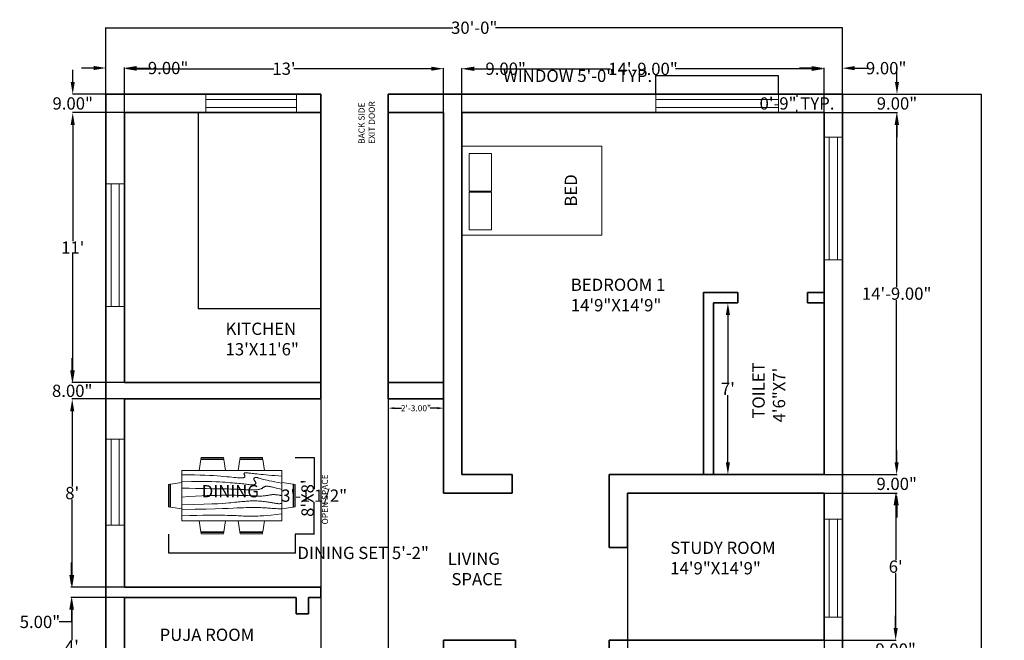
# Model space of a CAD drawing. Units: inches. Extents: x 14 to 1508, y -30 to 806.
# Tile 2 of 4: x 14 to 495, y 502 to 806. Entities that reach past the tile are written whole.
import ezdxf

# ---------------------------------------------------------------- set-up
doc = ezdxf.new("R2010")
doc.units = ezdxf.units.IN
doc.header["$MEASUREMENT"] = 0
for name, color, linetype, lineweight in [('A-ANNO-DIMS', 6, 'Continuous', 18), ('A-ANNO-TEXT', 7, 'Continuous', 18), ('A-AREA-IDEN', 3, 'Continuous', 18), ('A-FLOR-CASE', 8, 'Continuous', 25), ('A-FURN', 8, 'Continuous', 18), ('A-GLAZ', 4, 'Continuous', 18), ('A-WALL', 7, 'Continuous', 35)]:
    doc.layers.add(name, color=color, linetype=linetype, lineweight=lineweight)
doc.styles.get("Standard").update_dxf_attribs({"font": 'arial.ttf'})
doc.dimstyles.get("Standard").update_dxf_attribs({"dimtxt": 6, "dimasz": 0.18, "dimexe": 0.18, "dimexo": 0.0625, "dimgap": 0.09, "dimtad": 0, "dimtih": 1, "dimtoh": 1, "dimzin": 0, "dimdsep": 46, "dimlunit": 3, "dimtxsty": 'Standard', "dimcen": 0.09, "dimadec": 0, "dimazin": 0, "dimtfac": 1, "dimtofl": 0, "dimtmove": 0, "dimatfit": 3, "dimfxl": 1, "dimtolj": 1, "dimtzin": 0, "dimarcsym": 0})

# ---------------------------------------------------------------- blocks, each defined once
blk = doc.blocks.new('Dining Set - 36 x 72 in.')
for p, q in [((-22.2343, 26.00059), (-23.4847, 17.99762)), ((-22.2304, 26), (-5.7608, 26)), ((-22, 27.5), (-22.1562, 26.50042)), ((-5.8416, 26.5), (-22.1534, 26.5)), ((-22, 27.5), (-6, 27.5)), ((-5.8437, 26.49966), (-6, 27.5)), ((-4.5152, 17.99762), (-5.7655, 25.99926)), ((5.7657, 26.00059), (4.5153, 17.99762)), ((5.7696, 26), (22.2392, 26)), ((6, 27.5), (5.8438, 26.50042)), ((22.1584, 26.5), (5.8466, 26.5)), ((6, 27.5), (22, 27.5)), ((22.1563, 26.49966), (22, 27.5)), ((23.4848, 17.99762), (22.2345, 25.99926)), ((36, 18), (-36, 18)), ((-36, 18), (-36, -18)), ((36, -18), (36, 18)), ((-45.5, 8), (-44.5004, 8.15617)), ((-45.5, 8), (-45.5, -8)), ((-44.5, -8.15843), (-44.5, 8.15338)), ((-44.0006, 8.23428), (-35.9976, 9.48474)), ((-44, 8.23041), (-44, -8.23915)), ((44.0006, 8.23428), (35.9976, 9.48474)), ((44, 8.23041), (44, -8.23915)), ((44.5, -8.15843), (44.5, 8.15338)), ((45.5, 8), (44.5005, 8.15617)), ((45.5, 8), (45.5, -8)), ((-44.4997, -8.15631), (-45.5, -8)), ((-35.9976, -9.48476), (-43.9993, -8.2345)), ((35.9976, -9.48476), (43.9993, -8.2345)), ((44.4997, -8.15631), (45.5, -8)), ((-36, -18), (36, -18)), ((-22.2343, -26.0006), (-23.4847, -17.99762)), ((-4.5152, -17.99762), (-5.7655, -25.99928)), ((5.7657, -26.0006), (4.5153, -17.99762)), ((23.4848, -17.99762), (22.2345, -25.99928)), ((-22.2304, -26), (-5.7608, -26)), ((-22, -27.5), (-22.1562, -26.50044)), ((-5.8416, -26.5), (-22.1534, -26.5)), ((-22, -27.5), (-6, -27.5)), ((-5.8437, -26.49967), (-6, -27.5)), ((5.7696, -26), (22.2392, -26)), ((6, -27.5), (5.8438, -26.50044)), ((22.1584, -26.5), (5.8466, -26.5)), ((6, -27.5), (22, -27.5)), ((22.1563, -26.49967), (22, -27.5))]:
    blk.add_line(p, q)
for points in [[(-36, 15), (-31.1772, 14.97754), (-26.8079, 14.91406), (-22.8538, 14.81543), (-19.276, 14.6875), (-16.0362, 14.53613), (-13.0957, 14.36718), (-10.4159, 14.18652), (-7.9583, 14), (-5.6904, 13.81315), (-3.6035, 13.63021), (-1.6954, 13.45508), (0.0365, 13.29166), (1.5945, 13.14388), (2.9811, 13.01562), (4.1988, 12.9108), (5.25, 12.83333), (6.1393, 12.78613), (6.8802, 12.76823), (7.4883, 12.77767), (7.9792, 12.8125), (8.3685, 12.87077), (8.6719, 12.95052), (8.9049, 13.0498), (9.0833, 13.16666), (9.2205, 13.29899), (9.3216, 13.44401), (9.3895, 13.59879), (9.4271, 13.76041), (9.4373, 13.92594), (9.4232, 14.09245), (9.3875, 14.257), (9.3333, 14.41666), (9.2638, 14.56917), (9.1836, 14.71484), (9.0975, 14.85465), (9.0104, 14.98958), (8.9272, 15.1206), (8.8529, 15.2487), (8.7922, 15.37483), (8.75, 15.5), (8.7305, 15.62467), (8.7344, 15.74739), (8.7617, 15.86621), (8.8125, 15.97916), (8.8867, 16.08431), (8.9844, 16.17968), (9.1055, 16.26334), (9.25, 16.33333), (9.4189, 16.38802), (9.6172, 16.42708), (9.8506, 16.45052), (10.125, 16.45833), (10.4463, 16.45052), (10.8203, 16.42708), (11.2529, 16.38802), (11.75, 16.33333), (12.3184, 16.26318), (12.9694, 16.17838), (13.7151, 16.07991), (14.5677, 15.96875), (15.5395, 15.84586), (16.6426, 15.71224), (17.8893, 15.56884), (19.2917, 15.41666), (20.859, 15.25667), (22.5879, 15.08984), (24.4721, 14.91715), (26.5052, 14.73958), (28.6809, 14.5581), (30.9929, 14.3737), (33.4347, 14.18733), (36, 14)], [(-36, 10), (-28.9766, 10.14274), (-23.1725, 10.20442), (-18.4241, 10.19775), (-14.5677, 10.13541), (-11.4399, 10.03011), (-8.877, 9.89453), (-6.7154, 9.74137), (-4.7917, 9.58333), (-2.9698, 9.43082), (-1.2246, 9.28515), (0.4415, 9.14534), (2.026, 9.01041), (3.5266, 8.87939), (4.9408, 8.7513), (6.266, 8.62516), (7.5, 8.5), (8.6411, 8.37549), (9.6914, 8.2539), (10.6538, 8.13818), (11.5312, 8.03125), (12.3267, 7.93603), (13.043, 7.85547), (13.6831, 7.79248), (14.25, 7.75), (14.7471, 7.7303), (15.1797, 7.73307), (15.5537, 7.75732), (15.875, 7.80208), (16.1494, 7.86637), (16.3828, 7.94922), (16.5811, 8.04964), (16.75, 8.16666), (16.8944, 8.29915), (17.0143, 8.44531), (17.1089, 8.60319), (17.1771, 8.77083), (17.218, 8.94629), (17.2305, 9.1276), (17.2137, 9.31282), (17.1667, 9.5), (17.0895, 9.6875), (16.987, 9.875), (16.8649, 10.0625), (16.7292, 10.25), (16.5856, 10.4375), (16.4401, 10.625), (16.2985, 10.8125), (16.1667, 11), (16.05, 11.18733), (15.9518, 11.3737), (15.8752, 11.5581), (15.8229, 11.73958), (15.798, 11.91715), (15.8034, 12.08984), (15.842, 12.25667), (15.9167, 12.41666), (16.0295, 12.56836), (16.1784, 12.70833), (16.3605, 12.83268), (16.5729, 12.9375), (16.8127, 13.01888), (17.0768, 13.07291), (17.3625, 13.0957), (17.6667, 13.08333), (17.9894, 13.03312), (18.3418, 12.94726), (18.7382, 12.82918), (19.1927, 12.68229), (19.7195, 12.51001), (20.3327, 12.31575), (21.0465, 12.10294), (21.875, 11.875), (22.8357, 11.63354), (23.959, 11.37304), (25.2786, 11.08618), (26.8282, 10.76562), (28.6414, 10.40405), (30.752, 9.99414), (33.1936, 9.52856), (36, 9)], [(-36, 5.5), (-30.7157, 5.3348), (-26.069, 5.20963), (-21.9946, 5.11767), (-18.4271, 5.05208), (-15.3009, 5.00602), (-12.5508, 4.97265), (-10.1112, 4.94515), (-7.9167, 4.91666), (-5.909, 4.88167), (-4.0586, 4.83984), (-2.3429, 4.79215), (-0.7396, 4.73958), (0.7739, 4.6831), (2.22, 4.6237), (3.6213, 4.56233), (5, 4.5), (6.373, 4.43782), (7.7344, 4.3776), (9.0723, 4.32129), (10.375, 4.27083), (11.6309, 4.22819), (12.8281, 4.19531), (13.9551, 4.17415), (15, 4.16666), (15.954, 4.17448), (16.819, 4.19791), (17.6001, 4.23698), (18.3021, 4.29166), (18.9299, 4.36198), (19.4883, 4.44791), (19.9823, 4.54948), (20.4167, 4.66666), (20.7969, 4.79899), (21.1302, 4.94401), (21.4245, 5.09879), (21.6875, 5.26041), (21.9271, 5.42594), (22.1511, 5.59245), (22.3672, 5.757), (22.5834, 5.91666), (22.8065, 6.06868), (23.0404, 6.21093), (23.2879, 6.34147), (23.5521, 6.45833), (23.8358, 6.55957), (24.142, 6.64323), (24.4735, 6.70735), (24.8334, 6.75), (25.2235, 6.76969), (25.642, 6.76692), (26.0858, 6.74267), (26.5521, 6.69791), (27.0379, 6.63362), (27.5404, 6.55078), (28.0565, 6.45036), (28.5834, 6.33333), (29.1242, 6.19987), (29.7071, 6.04687), (30.3661, 5.87044), (31.1354, 5.66666), (32.0493, 5.43164), (33.142, 5.16146), (34.4475, 4.85221), (36, 4.5)], [(-36, -1), (-30.7915, -0.6591), (-26.0195, -0.38216), (-21.6519, -0.16284), (-17.6563, 0.00521), (-14.0005, 0.12833), (-10.6523, 0.21289), (-7.5796, 0.26522), (-4.75, 0.29166), (-2.134, 0.29793), (0.2878, 0.28711), (2.5317, 0.26163), (4.6146, 0.22396), (6.5529, 0.17651), (8.3633, 0.12174), (10.0623, 0.06209), (11.6667, 0), (13.1899, -0.06201), (14.6341, -0.1211), (15.9982, -0.17432), (17.2813, -0.21875), (18.4823, -0.25147), (19.6003, -0.26953), (20.6343, -0.27002), (21.5834, -0.25), (22.4481, -0.20768), (23.2357, -0.14584), (23.9549, -0.06836), (24.6146, 0.02083), (25.2235, 0.11784), (25.7904, 0.21875), (26.3241, 0.31966), (26.8334, 0.41666), (27.3265, 0.50618), (27.8099, 0.58593), (28.2894, 0.65397), (28.7709, 0.70833), (29.2601, 0.74707), (29.763, 0.76823), (30.2855, 0.76985), (30.8334, 0.75), (31.4088, 0.70784), (31.9994, 0.64713), (32.589, 0.57275), (33.1615, 0.48958), (33.7008, 0.4025), (34.1908, 0.3164), (34.6153, 0.23616), (34.9584, 0.16666), (35.2099, 0.11165), (35.3848, 0.07031), (35.504, 0.04069), (35.5886, 0.02083), (35.6594, 0.00879), (35.7377, 0.0026), (35.8442, 0.00032), (36, 0)], [(-36, -6.5), (-27.1843, -6.31267), (-20.084, -6.1263), (-14.469, -5.9419), (-10.1094, -5.76042), (-6.7752, -5.58285), (-4.2363, -5.41016), (-2.2629, -5.24333), (-0.625, -5.08334), (0.8708, -4.93099), (2.2715, -4.78646), (3.5872, -4.64974), (4.8281, -4.52084), (6.0046, -4.39974), (7.127, -4.28646), (8.2053, -4.18099), (9.25, -4.08334), (10.2705, -3.99382), (11.2734, -3.91407), (12.2647, -3.84603), (13.25, -3.79167), (14.2354, -3.75293), (15.2266, -3.73177), (16.2295, -3.73015), (17.25, -3.75), (18.2912, -3.79248), (19.3451, -3.85547), (20.4009, -3.93604), (21.4479, -4.03125), (22.4754, -4.13819), (23.4727, -4.25391), (24.4289, -4.37549), (25.3334, -4.5), (26.1785, -4.62492), (26.9694, -4.74935), (27.7145, -4.87281), (28.4219, -4.99479), (29.1, -5.11483), (29.7572, -5.23242), (30.4016, -5.34709), (31.0417, -5.45834), (31.6837, -5.56437), (32.3262, -5.65821), (32.9658, -5.73153), (33.599, -5.77604), (34.2224, -5.78345), (34.8327, -5.74545), (35.4264, -5.65373), (36, -5.5)], [(-36, -10), (-26.4022, -9.81299), (-18.4675, -9.62891), (-11.9839, -9.45069), (-6.7396, -9.28125), (-2.5226, -9.12354), (0.8789, -8.98047), (3.6769, -8.85498), (6.0833, -8.75), (8.2767, -8.66765), (10.3021, -8.60677), (12.1712, -8.56543), (13.8958, -8.54167), (15.4876, -8.53353), (16.9583, -8.53907), (18.3197, -8.55632), (19.5834, -8.58334), (20.7616, -8.61841), (21.8685, -8.66081), (22.9188, -8.71004), (23.9271, -8.76563), (24.9081, -8.82707), (25.8763, -8.89388), (26.8465, -8.96558), (27.8334, -9.04167), (28.8474, -9.12118), (29.8828, -9.20117), (30.93, -9.27824), (31.9792, -9.34896), (33.0205, -9.40991), (34.0443, -9.45768), (35.0407, -9.48885), (36, -9.5)], [(-36, -14.5), (-30.0881, -14.33513), (-25.0332, -14.21224), (-20.7312, -14.12647), (-17.0781, -14.07292), (-13.97, -14.04671), (-11.3027, -14.04297), (-8.9724, -14.05681), (-6.875, -14.08334), (-4.9224, -14.11833), (-3.0905, -14.16016), (-1.3709, -14.20785), (0.2448, -14.26042), (1.7647, -14.3169), (3.1973, -14.3763), (4.5507, -14.43767), (5.8333, -14.5), (7.0554, -14.5621), (8.235, -14.62175), (9.3922, -14.67652), (10.5469, -14.72396), (11.7192, -14.76164), (12.929, -14.78711), (14.1965, -14.79794), (15.5417, -14.79167), (16.9933, -14.76424), (18.6152, -14.70508), (20.4804, -14.60197), (22.6615, -14.44271), (25.2312, -14.21509), (28.2624, -13.9069), (31.8277, -13.50594), (36, -13)]]:
    blk.add_lwpolyline(points)
blk = doc.blocks.new('*D3')
at = {"layer": 'A-ANNO-DIMS', "color": 0, "lineweight": -2, "transparency": 16777216}
for p, q in [((193.96, 620), (193.96, 615.39)), ((220.96, 620), (220.96, 615.39)), ((196.96, 615.57), (200.45, 615.57)), ((217.96, 615.57), (214.48, 615.57))]:
    blk.add_line(p, q, dxfattribs=at)
at = {"layer": 'A-ANNO-DIMS', "color": 0, "transparency": 16777216}
for points in [[(196.96, 616.07), (196.96, 615.07), (193.96, 615.57)], [(217.96, 616.07), (217.96, 615.07), (220.96, 615.57)]]:
    blk.add_solid(points, dxfattribs=at)
at = {"layer": 'Defpoints', "color": 0, "transparency": 16777216}
for p in [(193.96, 620.06), (220.96, 620.06), (220.96, 615.57)]:
    blk.add_point(p, dxfattribs=at)
at = {"layer": 'A-ANNO-DIMS', "color": 0, "transparency": 16777216, "insert": (207.46, 615.57), "char_height": 3, "attachment_point": 5}
blk.add_mtext('\\A1;2\'-3.00"', dxfattribs=at)
blk = doc.blocks.new('*D4')
at = {"layer": 'A-ANNO-DIMS', "color": 0, "lineweight": -2, "transparency": 16777216}
for p, q in [((39.7, 775.06), (39.7, 781.06)), ((66.46, 769.06), (39.52, 769.06)), ((64.9, 760.06), (39.52, 760.06)), ((39.7, 754.06), (39.7, 748.06))]:
    blk.add_line(p, q, dxfattribs=at)
at = {"layer": 'A-ANNO-DIMS', "color": 0, "transparency": 16777216}
for points in [[(38.7, 775.06), (40.7, 775.06), (39.7, 769.06)], [(38.7, 754.06), (40.7, 754.06), (39.7, 760.06)]]:
    blk.add_solid(points, dxfattribs=at)
at = {"layer": 'Defpoints', "color": 0, "transparency": 16777216}
for p in [(66.52, 769.06), (39.7, 760.06), (64.96, 760.06)]:
    blk.add_point(p, dxfattribs=at)
at = {"layer": 'A-ANNO-DIMS', "color": 0, "transparency": 16777216, "insert": (39.7, 764.56), "char_height": 6, "attachment_point": 5}
blk.add_mtext('\\A1;9.00"', dxfattribs=at)
blk = doc.blocks.new('*D5')
at = {"layer": 'A-ANNO-DIMS', "color": 0, "lineweight": -2, "transparency": 16777216}
for p, q in [((64.9, 760.06), (39.52, 760.06)), ((39.7, 754.06), (39.7, 697.16)), ((39.7, 634.06), (39.7, 690.96)), ((64.9, 628.06), (39.52, 628.06))]:
    blk.add_line(p, q, dxfattribs=at)
at = {"layer": 'A-ANNO-DIMS', "color": 0, "transparency": 16777216}
for points in [[(38.7, 754.06), (40.7, 754.06), (39.7, 760.06)], [(38.7, 634.06), (40.7, 634.06), (39.7, 628.06)]]:
    blk.add_solid(points, dxfattribs=at)
at = {"layer": 'Defpoints', "color": 0, "transparency": 16777216}
for p in [(39.7, 760.06), (64.96, 760.06), (64.96, 628.06)]:
    blk.add_point(p, dxfattribs=at)
at = {"layer": 'A-ANNO-DIMS', "color": 0, "transparency": 16777216, "insert": (39.7, 694.06), "char_height": 6, "attachment_point": 5}
blk.add_mtext("\\A1;11'", dxfattribs=at)
blk = doc.blocks.new('*D6')
at = {"layer": 'A-ANNO-DIMS', "color": 0, "lineweight": -2, "transparency": 16777216}
for p, q in [((39.45, 634.06), (39.45, 640.06)), ((64.9, 628.06), (39.27, 628.06)), ((64.9, 620.06), (39.27, 620.06)), ((39.45, 614.06), (39.45, 608.06))]:
    blk.add_line(p, q, dxfattribs=at)
at = {"layer": 'A-ANNO-DIMS', "color": 0, "transparency": 16777216}
for points in [[(38.45, 634.06), (40.45, 634.06), (39.45, 628.06)], [(38.45, 614.06), (40.45, 614.06), (39.45, 620.06)]]:
    blk.add_solid(points, dxfattribs=at)
at = {"layer": 'Defpoints', "color": 0, "transparency": 16777216}
for p in [(64.96, 628.06), (39.45, 620.06), (64.96, 620.06)]:
    blk.add_point(p, dxfattribs=at)
at = {"layer": 'A-ANNO-DIMS', "color": 0, "transparency": 16777216, "insert": (39.45, 624.06), "char_height": 6, "attachment_point": 5}
blk.add_mtext('\\A1;8.00"', dxfattribs=at)
blk = doc.blocks.new('*D7')
at = {"layer": 'A-ANNO-DIMS', "color": 0, "lineweight": -2, "transparency": 16777216}
for p, q in [((64.9, 620.06), (39.27, 620.06)), ((39.45, 614.06), (39.45, 577.22)), ((39.45, 534.06), (39.45, 570.91)), ((64.9, 528.06), (39.27, 528.06))]:
    blk.add_line(p, q, dxfattribs=at)
at = {"layer": 'A-ANNO-DIMS', "color": 0, "transparency": 16777216}
for points in [[(38.45, 614.06), (40.45, 614.06), (39.45, 620.06)], [(38.45, 534.06), (40.45, 534.06), (39.45, 528.06)]]:
    blk.add_solid(points, dxfattribs=at)
at = {"layer": 'Defpoints', "color": 0, "transparency": 16777216}
for p in [(64.96, 620.06), (39.45, 528.06), (64.96, 528.06)]:
    blk.add_point(p, dxfattribs=at)
at = {"layer": 'A-ANNO-DIMS', "color": 0, "transparency": 16777216, "insert": (39.45, 574.06), "char_height": 6, "attachment_point": 5}
blk.add_mtext("\\A1;8'", dxfattribs=at)
blk = doc.blocks.new('*D8')
at = {"layer": 'A-ANNO-DIMS', "color": 0, "lineweight": -2, "transparency": 16777216}
for p, q in [((39.03, 534.06), (39.03, 540.06)), ((64.9, 528.06), (38.85, 528.06)), ((64.9, 523.06), (38.85, 523.06)), ((39.03, 517.06), (39.03, 511.06)), ((39.03, 511.06), (33.03, 511.06))]:
    blk.add_line(p, q, dxfattribs=at)
at = {"layer": 'A-ANNO-DIMS', "color": 0, "transparency": 16777216}
for points in [[(38.03, 534.06), (40.03, 534.06), (39.03, 528.06)], [(38.03, 517.06), (40.03, 517.06), (39.03, 523.06)]]:
    blk.add_solid(points, dxfattribs=at)
at = {"layer": 'Defpoints', "color": 0, "transparency": 16777216}
for p in [(64.96, 528.06), (39.03, 523.06), (64.96, 523.06)]:
    blk.add_point(p, dxfattribs=at)
at = {"layer": 'A-ANNO-DIMS', "color": 0, "transparency": 16777216, "insert": (23.67, 511.06), "char_height": 6, "attachment_point": 5}
blk.add_mtext('\\A1;5.00"', dxfattribs=at)
blk = doc.blocks.new('*D9')
at = {"layer": 'A-ANNO-DIMS', "color": 0, "lineweight": -2, "transparency": 16777216}
for p, q in [((64.9, 523.06), (39.11, 523.06)), ((39.29, 517.06), (39.29, 502.15)), ((39.29, 481.06), (39.29, 495.97)), ((64.9, 475.06), (39.11, 475.06))]:
    blk.add_line(p, q, dxfattribs=at)
at = {"layer": 'A-ANNO-DIMS', "color": 0, "transparency": 16777216}
for points in [[(38.29, 517.06), (40.29, 517.06), (39.29, 523.06)], [(38.29, 481.06), (40.29, 481.06), (39.29, 475.06)]]:
    blk.add_solid(points, dxfattribs=at)
at = {"layer": 'Defpoints', "color": 0, "transparency": 16777216}
for p in [(64.96, 523.06), (39.29, 475.06), (64.96, 475.06)]:
    blk.add_point(p, dxfattribs=at)
at = {"layer": 'A-ANNO-DIMS', "color": 0, "transparency": 16777216, "insert": (39.29, 499.06), "char_height": 6, "attachment_point": 5}
blk.add_mtext("\\A1;4'", dxfattribs=at)
blk = doc.blocks.new('*D15')
at = {"layer": 'A-ANNO-DIMS', "color": 0, "lineweight": -2, "transparency": 16777216}
for p, q in [((49.96, 781.88), (43.96, 781.88)), ((55.96, 760.12), (55.96, 782.06)), ((64.96, 760.12), (64.96, 782.06)), ((70.96, 781.88), (76.96, 781.88))]:
    blk.add_line(p, q, dxfattribs=at)
at = {"layer": 'A-ANNO-DIMS', "color": 0, "transparency": 16777216}
for points in [[(49.96, 782.88), (49.96, 780.88), (55.96, 781.88)], [(70.96, 782.88), (70.96, 780.88), (64.96, 781.88)]]:
    blk.add_solid(points, dxfattribs=at)
at = {"layer": 'Defpoints', "color": 0, "transparency": 16777216}
for p in [(64.96, 781.88), (55.96, 760.06), (64.96, 760.06)]:
    blk.add_point(p, dxfattribs=at)
at = {"layer": 'A-ANNO-DIMS', "color": 0, "transparency": 16777216, "insert": (86.33, 781.88), "char_height": 6, "attachment_point": 5}
blk.add_mtext('\\A1;9.00"', dxfattribs=at)
blk = doc.blocks.new('*D16')
at = {"layer": 'A-ANNO-DIMS', "color": 0, "lineweight": -2, "transparency": 16777216}
for p, q in [((64.96, 760.12), (64.96, 781.73)), ((70.96, 781.55), (138.06, 781.55)), ((214.96, 781.55), (147.86, 781.55)), ((220.96, 760.12), (220.96, 781.73))]:
    blk.add_line(p, q, dxfattribs=at)
at = {"layer": 'A-ANNO-DIMS', "color": 0, "transparency": 16777216}
for points in [[(70.96, 782.55), (70.96, 780.55), (64.96, 781.55)], [(214.96, 782.55), (214.96, 780.55), (220.96, 781.55)]]:
    blk.add_solid(points, dxfattribs=at)
at = {"layer": 'Defpoints', "color": 0, "transparency": 16777216}
for p in [(220.96, 781.55), (64.96, 760.06), (220.96, 760.06)]:
    blk.add_point(p, dxfattribs=at)
at = {"layer": 'A-ANNO-DIMS', "color": 0, "transparency": 16777216, "insert": (142.96, 781.55), "char_height": 6, "attachment_point": 5}
blk.add_mtext("\\A1;13'", dxfattribs=at)
blk = doc.blocks.new('*D17')
at = {"layer": 'A-ANNO-DIMS', "color": 0, "lineweight": -2, "transparency": 16777216}
for p, q in [((214.96, 781.55), (208.96, 781.55)), ((220.96, 760.12), (220.96, 781.73)), ((229.96, 760.12), (229.96, 781.73)), ((235.96, 781.55), (241.96, 781.55))]:
    blk.add_line(p, q, dxfattribs=at)
at = {"layer": 'A-ANNO-DIMS', "color": 0, "transparency": 16777216}
for points in [[(214.96, 782.55), (214.96, 780.55), (220.96, 781.55)], [(235.96, 782.55), (235.96, 780.55), (229.96, 781.55)]]:
    blk.add_solid(points, dxfattribs=at)
at = {"layer": 'Defpoints', "color": 0, "transparency": 16777216}
for p in [(229.96, 781.55), (220.96, 760.06), (229.96, 760.06)]:
    blk.add_point(p, dxfattribs=at)
at = {"layer": 'A-ANNO-DIMS', "color": 0, "transparency": 16777216, "insert": (251.33, 781.55), "char_height": 6, "attachment_point": 5}
blk.add_mtext('\\A1;9.00"', dxfattribs=at)
blk = doc.blocks.new('*D18')
at = {"layer": 'A-ANNO-DIMS', "color": 0, "lineweight": -2, "transparency": 16777216}
for p, q in [((229.96, 760.12), (229.96, 781.64)), ((235.96, 781.46), (302.52, 781.46)), ((400.96, 781.46), (334.4, 781.46)), ((406.96, 760.12), (406.96, 781.64))]:
    blk.add_line(p, q, dxfattribs=at)
at = {"layer": 'A-ANNO-DIMS', "color": 0, "transparency": 16777216}
for points in [[(235.96, 782.46), (235.96, 780.46), (229.96, 781.46)], [(400.96, 782.46), (400.96, 780.46), (406.96, 781.46)]]:
    blk.add_solid(points, dxfattribs=at)
at = {"layer": 'Defpoints', "color": 0, "transparency": 16777216}
for p in [(406.96, 781.46), (229.96, 760.06), (406.96, 760.06)]:
    blk.add_point(p, dxfattribs=at)
at = {"layer": 'A-ANNO-DIMS', "color": 0, "transparency": 16777216, "insert": (318.46, 781.46), "char_height": 6, "attachment_point": 5}
blk.add_mtext('\\A1;14\'-9.00"', dxfattribs=at)
blk = doc.blocks.new('*D19')
at = {"layer": 'A-ANNO-DIMS', "color": 0, "lineweight": -2, "transparency": 16777216}
for p, q in [((400.96, 781.81), (394.96, 781.81)), ((406.96, 769.12), (406.96, 781.99)), ((415.96, 769.12), (415.96, 781.99)), ((421.96, 781.81), (427.96, 781.81))]:
    blk.add_line(p, q, dxfattribs=at)
at = {"layer": 'A-ANNO-DIMS', "color": 0, "transparency": 16777216}
for points in [[(400.96, 782.81), (400.96, 780.81), (406.96, 781.81)], [(421.96, 782.81), (421.96, 780.81), (415.96, 781.81)]]:
    blk.add_solid(points, dxfattribs=at)
at = {"layer": 'Defpoints', "color": 0, "transparency": 16777216}
for p in [(415.96, 781.81), (406.96, 769.06), (415.96, 769.06)]:
    blk.add_point(p, dxfattribs=at)
at = {"layer": 'A-ANNO-DIMS', "color": 0, "transparency": 16777216, "insert": (437.33, 781.81), "char_height": 6, "attachment_point": 5}
blk.add_mtext('\\A1;9.00"', dxfattribs=at)
blk = doc.blocks.new('*D20')
at = {"layer": 'A-ANNO-DIMS', "color": 0, "lineweight": -2, "transparency": 16777216}
for p, q in [((442.61, 775.06), (442.61, 781.06)), ((407.03, 769.06), (442.79, 769.06)), ((407.03, 760.06), (442.79, 760.06)), ((442.61, 754.06), (442.61, 748.06))]:
    blk.add_line(p, q, dxfattribs=at)
at = {"layer": 'A-ANNO-DIMS', "color": 0, "transparency": 16777216}
for points in [[(441.61, 775.06), (443.61, 775.06), (442.61, 769.06)], [(441.61, 754.06), (443.61, 754.06), (442.61, 760.06)]]:
    blk.add_solid(points, dxfattribs=at)
at = {"layer": 'Defpoints', "color": 0, "transparency": 16777216}
for p in [(406.96, 769.06), (406.96, 760.06), (442.61, 760.06)]:
    blk.add_point(p, dxfattribs=at)
at = {"layer": 'A-ANNO-DIMS', "color": 0, "transparency": 16777216, "insert": (442.61, 764.56), "char_height": 6, "attachment_point": 5}
blk.add_mtext('\\A1;9.00"', dxfattribs=at)
blk = doc.blocks.new('*D21')
at = {"layer": 'A-ANNO-DIMS', "color": 0, "lineweight": -2, "transparency": 16777216}
for p, q in [((407.03, 760.06), (442.63, 760.06)), ((442.45, 754.06), (442.45, 674.72)), ((442.45, 589.06), (442.45, 668.41)), ((407.03, 583.06), (442.63, 583.06))]:
    blk.add_line(p, q, dxfattribs=at)
at = {"layer": 'A-ANNO-DIMS', "color": 0, "transparency": 16777216}
for points in [[(441.45, 754.06), (443.45, 754.06), (442.45, 760.06)], [(441.45, 589.06), (443.45, 589.06), (442.45, 583.06)]]:
    blk.add_solid(points, dxfattribs=at)
at = {"layer": 'Defpoints', "color": 0, "transparency": 16777216}
for p in [(406.96, 760.06), (406.96, 583.06), (442.45, 583.06)]:
    blk.add_point(p, dxfattribs=at)
at = {"layer": 'A-ANNO-DIMS', "color": 0, "transparency": 16777216, "insert": (442.45, 671.56), "char_height": 6, "attachment_point": 5}
blk.add_mtext('\\A1;14\'-9.00"', dxfattribs=at)
blk = doc.blocks.new('*D22')
at = {"layer": 'A-ANNO-DIMS', "color": 0, "lineweight": -2, "transparency": 16777216}
for p, q in [((442.47, 589.06), (442.47, 595.06)), ((407.03, 583.06), (442.65, 583.06)), ((407.03, 574.06), (442.65, 574.06)), ((442.47, 568.06), (442.47, 562.06))]:
    blk.add_line(p, q, dxfattribs=at)
at = {"layer": 'A-ANNO-DIMS', "color": 0, "transparency": 16777216}
for points in [[(441.47, 589.06), (443.47, 589.06), (442.47, 583.06)], [(441.47, 568.06), (443.47, 568.06), (442.47, 574.06)]]:
    blk.add_solid(points, dxfattribs=at)
at = {"layer": 'Defpoints', "color": 0, "transparency": 16777216}
for p in [(406.96, 583.06), (406.96, 574.06), (442.47, 574.06)]:
    blk.add_point(p, dxfattribs=at)
at = {"layer": 'A-ANNO-DIMS', "color": 0, "transparency": 16777216, "insert": (442.47, 578.56), "char_height": 6, "attachment_point": 5}
blk.add_mtext('\\A1;9.00"', dxfattribs=at)
blk = doc.blocks.new('*D23')
at = {"layer": 'A-ANNO-DIMS', "color": 0, "lineweight": -2, "transparency": 16777216}
for p, q in [((407.03, 574.06), (442.16, 574.06)), ((441.98, 568.06), (441.98, 541.22)), ((441.98, 508.06), (441.98, 534.91)), ((407.03, 502.06), (442.16, 502.06))]:
    blk.add_line(p, q, dxfattribs=at)
at = {"layer": 'A-ANNO-DIMS', "color": 0, "transparency": 16777216}
for points in [[(440.98, 568.06), (442.98, 568.06), (441.98, 574.06)], [(440.98, 508.06), (442.98, 508.06), (441.98, 502.06)]]:
    blk.add_solid(points, dxfattribs=at)
at = {"layer": 'Defpoints', "color": 0, "transparency": 16777216}
for p in [(406.96, 574.06), (406.96, 502.06), (441.98, 502.06)]:
    blk.add_point(p, dxfattribs=at)
at = {"layer": 'A-ANNO-DIMS', "color": 0, "transparency": 16777216, "insert": (441.98, 538.06), "char_height": 6, "attachment_point": 5}
blk.add_mtext("\\A1;6'", dxfattribs=at)
blk = doc.blocks.new('*D24')
at = {"layer": 'A-ANNO-DIMS', "color": 0, "lineweight": -2, "transparency": 16777216}
for p, q in [((441.97, 508.06), (441.97, 514.06)), ((407.03, 502.06), (442.15, 502.06)), ((407.03, 493.06), (442.15, 493.06)), ((441.97, 487.06), (441.97, 481.06))]:
    blk.add_line(p, q, dxfattribs=at)
at = {"layer": 'A-ANNO-DIMS', "color": 0, "transparency": 16777216}
for points in [[(440.97, 508.06), (442.97, 508.06), (441.97, 502.06)], [(440.97, 487.06), (442.97, 487.06), (441.97, 493.06)]]:
    blk.add_solid(points, dxfattribs=at)
at = {"layer": 'Defpoints', "color": 0, "transparency": 16777216}
for p in [(406.96, 502.06), (406.96, 493.06), (441.97, 493.06)]:
    blk.add_point(p, dxfattribs=at)
at = {"layer": 'A-ANNO-DIMS', "color": 0, "transparency": 16777216, "insert": (441.97, 497.56), "char_height": 6, "attachment_point": 5}
blk.add_mtext('\\A1;9.00"', dxfattribs=at)
blk = doc.blocks.new('*D27')
at = {"layer": 'A-ANNO-DIMS', "color": 0, "lineweight": -2, "transparency": 16777216}
for p, q in [((353.03, 667.06), (360.14, 667.06)), ((359.96, 661.06), (359.96, 628.15)), ((359.96, 589.06), (359.96, 621.97)), ((353.03, 583.06), (360.14, 583.06))]:
    blk.add_line(p, q, dxfattribs=at)
at = {"layer": 'A-ANNO-DIMS', "color": 0, "transparency": 16777216}
for points in [[(358.96, 661.06), (360.96, 661.06), (359.96, 667.06)], [(358.96, 589.06), (360.96, 589.06), (359.96, 583.06)]]:
    blk.add_solid(points, dxfattribs=at)
at = {"layer": 'Defpoints', "color": 0, "transparency": 16777216}
for p in [(352.96, 667.06), (352.96, 583.06), (359.96, 583.06)]:
    blk.add_point(p, dxfattribs=at)
at = {"layer": 'A-ANNO-DIMS', "color": 0, "transparency": 16777216, "insert": (359.96, 625.06), "char_height": 6, "attachment_point": 5}
blk.add_mtext("\\A1;7'", dxfattribs=at)
blk = doc.blocks.new('WIN-60IN')
for p, q in [((0, 60), (9, 60)), ((2.5, 0), (2.5, 60)), ((6.5, 0), (6.5, 60)), ((0, 0), (9, 0))]:
    blk.add_line(p, q)
blk = doc.blocks.new('WIN-48IN')
for p, q in [((0, 48), (9, 48)), ((2.5, 48), (2.5, 0)), ((6.5, 48), (6.5, 0)), ((0, 0), (9, 0))]:
    blk.add_line(p, q)
blk = doc.blocks.new('*D87')
at = {"layer": 'A-ANNO-DIMS', "color": 0, "lineweight": -2, "transparency": 16777216}
for p, q in [((324.74, 778.06), (324.56, 778.06)), ((324.74, 769.12), (324.74, 778.24)), ((384.56, 778.06), (324.92, 778.06)), ((384.74, 769.12), (384.74, 778.24))]:
    blk.add_line(p, q, dxfattribs=at)
at = {"layer": 'A-ANNO-DIMS', "color": 0, "transparency": 16777216}
for points in [[(324.92, 778.09), (324.92, 778.03), (324.74, 778.06)], [(384.56, 778.09), (384.56, 778.03), (384.74, 778.06)]]:
    blk.add_solid(points, dxfattribs=at)
at = {"layer": 'Defpoints', "color": 0, "transparency": 16777216}
for p in [(324.74, 778.06), (324.74, 769.06), (384.74, 769.06)]:
    blk.add_point(p, dxfattribs=at)
at = {"layer": 'A-ANNO-DIMS', "color": 0, "transparency": 16777216, "insert": (286.51, 778.06), "char_height": 6, "attachment_point": 5}
blk.add_mtext('\\A1;WINDOW 5\'-0" TYP.', dxfattribs=at)
blk = doc.blocks.new('*D88')
at = {"layer": 'A-ANNO-DIMS', "color": 0, "lineweight": -2, "transparency": 16777216}
for p, q in [((384.81, 769.06), (393.92, 769.06)), ((393.74, 768.88), (393.74, 767.72)), ((393.74, 760.24), (393.74, 761.41)), ((384.81, 760.06), (393.92, 760.06))]:
    blk.add_line(p, q, dxfattribs=at)
at = {"layer": 'A-ANNO-DIMS', "color": 0, "transparency": 16777216}
for points in [[(393.71, 768.88), (393.77, 768.88), (393.74, 769.06)], [(393.71, 760.24), (393.77, 760.24), (393.74, 760.06)]]:
    blk.add_solid(points, dxfattribs=at)
at = {"layer": 'Defpoints', "color": 0, "transparency": 16777216}
for p in [(384.74, 769.06), (393.74, 769.06), (384.74, 760.06)]:
    blk.add_point(p, dxfattribs=at)
at = {"layer": 'A-ANNO-DIMS', "color": 0, "transparency": 16777216, "insert": (393.74, 764.56), "char_height": 6, "attachment_point": 5}
blk.add_mtext('\\A1;0\'-9" TYP.', dxfattribs=at)
blk = doc.blocks.new('*D95')
at = {"layer": 'A-ANNO-DIMS', "color": 0, "lineweight": -2, "transparency": 16777216}
for p, q in [((86.51, 554.02), (86.51, 544.61)), ((148.42, 554.02), (148.42, 544.61)), ((86.69, 544.79), (148.24, 544.79)), ((148.42, 544.79), (148.6, 544.79))]:
    blk.add_line(p, q, dxfattribs=at)
at = {"layer": 'A-ANNO-DIMS', "color": 0, "transparency": 16777216}
for points in [[(86.69, 544.82), (86.69, 544.76), (86.51, 544.79)], [(148.24, 544.82), (148.24, 544.76), (148.42, 544.79)]]:
    blk.add_solid(points, dxfattribs=at)
at = {"layer": 'Defpoints', "color": 0, "transparency": 16777216}
for p in [(86.51, 554.08), (148.42, 554.08), (148.42, 544.79)]:
    blk.add_point(p, dxfattribs=at)
at = {"layer": 'A-ANNO-DIMS', "color": 0, "transparency": 16777216, "insert": (181.67, 544.79), "char_height": 6, "attachment_point": 5}
blk.add_mtext('\\A1;DINING SET 5\'-2"', dxfattribs=at)
blk = doc.blocks.new('*D96')
at = {"layer": 'A-ANNO-DIMS', "color": 0, "lineweight": -2, "transparency": 16777216}
for p, q in [((148.49, 591.5), (157.89, 591.5)), ((157.71, 591.32), (157.71, 575.99)), ((157.71, 554.26), (157.71, 569.6)), ((148.49, 554.08), (157.89, 554.08))]:
    blk.add_line(p, q, dxfattribs=at)
at = {"layer": 'A-ANNO-DIMS', "color": 0, "transparency": 16777216}
for points in [[(157.68, 591.32), (157.74, 591.32), (157.71, 591.5)], [(157.68, 554.26), (157.74, 554.26), (157.71, 554.08)]]:
    blk.add_solid(points, dxfattribs=at)
at = {"layer": 'Defpoints', "color": 0, "transparency": 16777216}
for p in [(148.42, 591.5), (157.71, 591.5), (148.42, 554.08)]:
    blk.add_point(p, dxfattribs=at)
at = {"layer": 'A-ANNO-DIMS', "color": 0, "transparency": 16777216, "insert": (157.71, 572.79), "char_height": 6, "attachment_point": 5}
blk.add_mtext('\\A1;3\'-1 1/2"', dxfattribs=at)
blk = doc.blocks.new('*D98')
at = {"layer": 'A-ANNO-DIMS', "color": 0, "lineweight": -2, "transparency": 16777216}
for p, q in [((55.96, 769.12), (55.96, 801.76)), ((56.14, 801.58), (225.57, 801.58)), ((415.78, 801.58), (246.36, 801.58)), ((415.96, 769.12), (415.96, 801.76))]:
    blk.add_line(p, q, dxfattribs=at)
at = {"layer": 'A-ANNO-DIMS', "color": 0, "transparency": 16777216}
for points in [[(56.14, 801.61), (56.14, 801.55), (55.96, 801.58)], [(415.78, 801.61), (415.78, 801.55), (415.96, 801.58)]]:
    blk.add_solid(points, dxfattribs=at)
at = {"layer": 'Defpoints', "color": 0, "transparency": 16777216}
for p in [(415.96, 801.58), (55.96, 769.06), (415.96, 769.06)]:
    blk.add_point(p, dxfattribs=at)
at = {"layer": 'A-ANNO-DIMS', "color": 0, "transparency": 16777216, "insert": (235.96, 801.58), "char_height": 6, "attachment_point": 5}
blk.add_mtext('\\A1;30\'-0"', dxfattribs=at)
blk = doc.blocks.new('*D99')
at = {"layer": 'A-ANNO-DIMS', "color": 0, "lineweight": -2, "transparency": 16777216}
for p, q in [((416.03, 769.06), (483.95, 769.06)), ((483.77, 768.88), (483.77, 453.32)), ((483.77, 131.44), (483.77, 447)), ((451.31, 131.26), (483.95, 131.26))]:
    blk.add_line(p, q, dxfattribs=at)
at = {"layer": 'A-ANNO-DIMS', "color": 0, "transparency": 16777216}
for points in [[(483.74, 768.88), (483.8, 768.88), (483.77, 769.06)], [(483.74, 131.44), (483.8, 131.44), (483.77, 131.26)]]:
    blk.add_solid(points, dxfattribs=at)
at = {"layer": 'Defpoints', "color": 0, "transparency": 16777216}
for p in [(415.96, 769.06), (483.77, 769.06), (451.25, 131.26)]:
    blk.add_point(p, dxfattribs=at)
at = {"layer": 'A-ANNO-DIMS', "color": 0, "transparency": 16777216, "insert": (483.77, 450.16), "char_height": 6, "attachment_point": 5}
blk.add_mtext('\\A1;53\'-2"', dxfattribs=at)
blk = doc.blocks.new('*D100')
at = {"layer": 'A-ANNO-DIMS', "color": 0, "lineweight": -2, "transparency": 16777216}
for p, q in [((160.96, 760), (160.96, 98.56)), ((193.96, 760), (193.96, 98.56)), ((161.14, 98.74), (169.35, 98.74)), ((193.78, 98.74), (185.58, 98.74))]:
    blk.add_line(p, q, dxfattribs=at)
at = {"layer": 'A-ANNO-DIMS', "color": 0, "transparency": 16777216}
for points in [[(161.14, 98.77), (161.14, 98.71), (160.96, 98.74)], [(193.78, 98.77), (193.78, 98.71), (193.96, 98.74)]]:
    blk.add_solid(points, dxfattribs=at)
at = {"layer": 'Defpoints', "color": 0, "transparency": 16777216}
for p in [(160.96, 760.06), (193.96, 760.06), (160.96, 98.74)]:
    blk.add_point(p, dxfattribs=at)
at = {"layer": 'A-ANNO-DIMS', "color": 0, "transparency": 16777216, "insert": (177.46, 98.74), "char_height": 6, "attachment_point": 5}
blk.add_mtext('\\A1;2\'-9"', dxfattribs=at)
blk = doc.blocks.new('*D102')
at = {"layer": 'A-ANNO-DIMS', "color": 0, "lineweight": -2, "transparency": 16777216}
for p, q in [((310.96, 574), (310.96, 98.56)), ((406.96, 574), (406.96, 98.56)), ((311.14, 98.74), (350.89, 98.74)), ((406.78, 98.74), (367.03, 98.74))]:
    blk.add_line(p, q, dxfattribs=at)
at = {"layer": 'A-ANNO-DIMS', "color": 0, "transparency": 16777216}
for points in [[(311.14, 98.77), (311.14, 98.71), (310.96, 98.74)], [(406.78, 98.77), (406.78, 98.71), (406.96, 98.74)]]:
    blk.add_solid(points, dxfattribs=at)
at = {"layer": 'Defpoints', "color": 0, "transparency": 16777216}
for p in [(310.96, 574.06), (406.96, 574.06), (406.96, 98.74)]:
    blk.add_point(p, dxfattribs=at)
at = {"layer": 'A-ANNO-DIMS', "color": 0, "transparency": 16777216, "insert": (358.96, 98.74), "char_height": 6, "attachment_point": 5}
blk.add_mtext('\\A1;8\'-0"', dxfattribs=at)

msp = doc.modelspace()

# ---------------------------------------------------------------- linework, layer by layer
at = {"layer": 'A-FLOR-CASE'}
for points in [[(100.963, 760.062), (100.963, 664.062)], [(160.963, 664.062), (100.963, 664.062)]]:
    msp.add_lwpolyline(points, dxfattribs=at)
at = {"layer": 'A-FURN'}
for points in [[(229.963, 743.637), (298.388, 743.637), (298.388, 700.077), (229.963, 700.077)], [(233.442, 740.035), (244.429, 740.035), (244.429, 721.629), (233.442, 721.629)], [(233.442, 721.145), (244.429, 721.145), (244.429, 702.739), (233.442, 702.739)]]:
    msp.add_lwpolyline(points, close=True, dxfattribs=at)
at = {"layer": 'A-GLAZ'}
for p, q in [((104.683, 769.062), (104.683, 760.062)), ((104.683, 766.562), (149.032, 766.562)), ((149.032, 769.062), (149.032, 760.062)), ((104.683, 762.562), (149.032, 762.562)), ((64.963, 600.432), (55.963, 600.432)), ((58.463, 558.432), (58.463, 600.432)), ((62.463, 558.432), (62.463, 600.432)), ((64.963, 558.432), (55.963, 558.432))]:
    msp.add_line(p, q, dxfattribs=at)
at = {"layer": 'A-WALL'}
for p, q in [((364.796, 672.062), (364.796, 667.062)), ((398.806, 672.062), (398.806, 667.062)), ((254.465, 583.062), (254.465, 574.062)), ((301.963, 547.396), (310.963, 547.396)), ((148.963, 515.018), (154.963, 515.018)), ((256.109, 502.062), (256.109, 493.062))]:
    msp.add_line(p, q, dxfattribs=at)
for points in [[(160.963, 769.062), (55.963, 769.062), (55.963, 169.062)], [(160.963, 769.062), (160.963, 620.062)], [(193.963, 769.062), (193.963, 620.062)], [(415.963, 304.062), (415.963, 769.062), (193.963, 769.062)], [(64.963, 760.062), (64.963, 628.062)], [(160.963, 760.062), (64.963, 760.062)], [(220.963, 760.062), (193.963, 760.062)], [(220.963, 760.062), (220.963, 574.062)], [(406.963, 760.062), (229.963, 760.062)], [(229.963, 583.062), (229.963, 760.062)], [(406.963, 583.062), (406.963, 760.062)], [(347.963, 583.062), (347.963, 672.062), (364.796, 672.062)], [(398.806, 672.062), (406.963, 672.062)], [(364.796, 667.062), (352.963, 667.062)], [(352.963, 583.062), (352.963, 667.062)], [(406.963, 667.062), (398.806, 667.062)], [(160.963, 628.062), (64.963, 628.062)], [(220.963, 628.062), (193.963, 628.062)], [(64.963, 620.062), (64.963, 528.062)], [(160.963, 620.062), (64.963, 620.062)], [(220.963, 620.062), (193.963, 620.062)], [(254.465, 583.062), (229.963, 583.062)], [(406.963, 583.062), (301.963, 583.062)], [(301.963, 547.396), (301.963, 583.062)], [(254.465, 574.062), (220.963, 574.062)], [(406.963, 574.062), (310.963, 574.062)], [(310.963, 547.396), (310.963, 574.062)], [(406.963, 502.062), (406.963, 574.062)], [(64.963, 528.062), (160.963, 528.062)], [(160.963, 528.062), (160.963, 523.062)], [(64.963, 523.062), (148.963, 523.062)], [(64.963, 523.062), (64.963, 475.062)], [(148.963, 523.062), (148.963, 515.018)], [(154.963, 523.062), (154.963, 515.018)], [(154.963, 523.062), (160.963, 523.062)], [(220.963, 502.062), (220.963, 469.062)], [(256.109, 502.062), (220.963, 502.062)], [(406.963, 502.062), (301.963, 502.062)], [(301.963, 493.062), (301.963, 502.062)]]:
    msp.add_lwpolyline(points, dxfattribs=at)

# ---------------------------------------------------------------- block references
at = {"layer": 'A-FURN', "xscale": 0.6803646124637545, "yscale": 0.6803646124637545, "zscale": 0.6803646124637545}
msp.add_blockref('Dining Set - 36 x 72 in.', (117.468, 572.792), dxfattribs=at)
at = {"layer": 'A-GLAZ', "rotation": 89.99999999999991}
msp.add_blockref('WIN-60IN', (384.743, 760.062), dxfattribs=at)
at = {"layer": 'A-GLAZ'}
for name, p in [('WIN-60IN', (406.963, 688.035)), ('WIN-60IN', (55.963, 665.227)), ('WIN-48IN', (406.963, 513.33))]:
    msp.add_blockref(name, p, dxfattribs=at)

# ---------------------------------------------------------------- texts
at = {"layer": 'A-ANNO-TEXT', "char_height": 6, "attachment_point": 1, "rotation": 90}
for s, insert in [('\\P{\\H0.5x;BACK SIDE\\PEXIT DOOR}', (169.379, 744.8)), ('BED', (280.223, 714.101))]:
    msp.add_mtext_dynamic_manual_height_columns(s, width=241.93696, gutter_width=1, heights=[0], dxfattribs=dict(at, insert=insert))
at = {"layer": 'A-AREA-IDEN', "char_height": 6, "attachment_point": 1}
for s, insert in [('BEDROOM 1\\P14\'9"X14\'9"', (283.171, 678.914)), ('KITCHEN\\P13\'X11\'6"', (114.41, 657.382)), ('DINING', (102.773, 577.966)), ('STUDY ROOM \\P14\'9"X14\'9"', (331.796, 550.288)), ('LIVING\\P SPACE ', (222.987, 544.96)), ("PUJA ROOM\\P        7'X4'", (82.167, 507.758))]:
    msp.add_mtext_dynamic_manual_height_columns(s, width=241.93696, gutter_width=1, heights=[0], dxfattribs=dict(at, insert=insert))
at = {"layer": 'A-AREA-IDEN', "char_height": 6, "attachment_point": 1, "rotation": 90}
for s, insert in [(' TOILET\\P4\'6"X7\'', (371.959, 608.599)), ("  8'X8'\\P{\\H0.5x;OPEN SPACE}", (151.488, 558.727))]:
    msp.add_mtext_dynamic_manual_height_columns(s, width=241.93696, gutter_width=1, heights=[0], dxfattribs=dict(at, insert=insert))

# ---------------------------------------------------------------- dimensions: what is measured, and where the dimension line sits
at = {"layer": 'A-ANNO-DIMS'}
for base, p1, p2, override, picture, middle in [((415.963, 801.577), (55.963, 769.062), (415.963, 769.062), {"dimdec": 1, "dimlfac": 1, "dimrnd": 0, "dimzin": 1, "dimdsep": 46, "dimlunit": 4, "dimfrac": 2}, '*D98', (235.963, 801.577)), ((64.963, 781.88), (55.963, 760.062), (64.963, 760.062), {"dimasz": 6, "dimclrd": 0, "dimclre": 0, "dimclrt": 0}, '*D15', (86.327, 781.88)), ((220.963, 781.552), (64.963, 760.062), (220.963, 760.062), {"dimasz": 6, "dimclrd": 0, "dimclre": 0, "dimclrt": 0}, '*D16', (142.963, 781.552)), ((229.963, 781.552), (220.963, 760.062), (229.963, 760.062), {"dimasz": 6, "dimclrd": 0, "dimclre": 0, "dimclrt": 0}, '*D17', (251.327, 781.552)), ((406.963, 781.459), (229.963, 760.062), (406.963, 760.062), {"dimasz": 6, "dimclrd": 0, "dimclre": 0, "dimclrt": 0}, '*D18', (318.463, 781.459)), ((415.963, 781.805), (406.963, 769.062), (415.963, 769.062), {"dimasz": 6, "dimclrd": 0, "dimclre": 0, "dimclrt": 0}, '*D19', (437.327, 781.805)), ((160.963, 98.743), (193.963, 760.062), (160.963, 760.062), {"dimdec": 1, "dimlfac": 1, "dimrnd": 0, "dimzin": 1, "dimdsep": 46, "dimlunit": 4, "dimfrac": 2}, '*D100', (177.463, 98.743)), ((220.963, 615.572), (193.963, 620.062), (220.963, 620.062), {"dimtxt": 3, "dimasz": 3, "dimclrd": 0, "dimclre": 0, "dimclrt": 0}, '*D3', (207.463, 615.572)), ((406.963, 98.743), (310.963, 574.062), (406.963, 574.062), {"dimdec": 1, "dimlfac": 1, "dimrnd": 0, "dimzin": 1, "dimdsep": 46, "dimlunit": 4, "dimfrac": 2}, '*D102', (358.963, 98.743))]:
    dim = msp.add_linear_dim(base=base, p1=p1, p2=p2, dimstyle='Standard', override=override, dxfattribs=at)
    dim.commit()
    dim.dimension.update_dxf_attribs({"geometry": picture, "text_midpoint": middle})
for base, p1, p2, angle, text, override, picture, middle in [((324.743, 778.062), (384.743, 769.062), (324.743, 769.062), 180, 'WINDOW <> TYP.', {"dimdec": 1, "dimlfac": 1, "dimrnd": 0, "dimzin": 1, "dimdsep": 46, "dimlunit": 4, "dimfrac": 2}, '*D87', (286.511, 778.062)), ((393.743, 769.062), (384.743, 760.062), (384.743, 769.062), 90, '<> TYP.', {"dimdec": 1, "dimlfac": 1, "dimrnd": 0, "dimzin": 1, "dimdsep": 46, "dimlunit": 4, "dimfrac": 2}, '*D88', (393.743, 764.562)), ((39.446, 528.062), (64.963, 620.062), (64.963, 528.062), 90, "8'", {"dimasz": 6, "dimclrd": 0, "dimclre": 0, "dimclrt": 0}, '*D7', (39.446, 574.062))]:
    dim = msp.add_linear_dim(base=base, p1=p1, p2=p2, angle=angle, text=text, dimstyle='Standard', override=override, dxfattribs=at)
    dim.commit()
    dim.dimension.update_dxf_attribs({"geometry": picture, "text_midpoint": middle})
for base, p1, p2, override, picture, middle in [((39.701, 760.062), (66.524, 769.062), (64.963, 760.062), {"dimasz": 6, "dimclrd": 0, "dimclre": 0, "dimclrt": 0}, '*D4', (39.701, 764.562)), ((442.606, 760.062), (406.963, 769.062), (406.963, 760.062), {"dimasz": 6, "dimclrd": 0, "dimclre": 0, "dimclrt": 0}, '*D20', (442.606, 764.562)), ((483.766, 769.062), (451.251, 131.258), (415.963, 769.062), {"dimdec": 1, "dimlfac": 1, "dimrnd": 0, "dimzin": 1, "dimdsep": 46, "dimlunit": 4, "dimfrac": 2}, '*D99', (483.766, 450.16)), ((39.701, 760.062), (64.963, 628.062), (64.963, 760.062), {"dimasz": 6, "dimclrd": 0, "dimclre": 0, "dimclrt": 0}, '*D5', (39.701, 694.062)), ((442.452, 583.062), (406.963, 760.062), (406.963, 583.062), {"dimasz": 6, "dimclrd": 0, "dimclre": 0, "dimclrt": 0}, '*D21', (442.452, 671.562)), ((359.963, 583.062), (352.963, 667.062), (352.963, 583.062), {"dimasz": 6, "dimclrd": 0, "dimclre": 0, "dimclrt": 0}, '*D27', (359.963, 625.062)), ((39.45, 620.062), (64.963, 628.062), (64.963, 620.062), {"dimasz": 6, "dimclrd": 0, "dimclre": 0, "dimclrt": 0}, '*D6', (39.45, 624.062)), ((442.47, 574.062), (406.963, 583.062), (406.963, 574.062), {"dimasz": 6, "dimclrd": 0, "dimclre": 0, "dimclrt": 0}, '*D22', (442.47, 578.562)), ((157.711, 591.502), (148.424, 554.082), (148.424, 591.502), {"dimdec": 1, "dimlfac": 1, "dimrnd": 0, "dimzin": 1, "dimdsep": 46, "dimlunit": 4, "dimfrac": 2}, '*D96', (157.711, 572.792)), ((441.982, 502.062), (406.963, 574.062), (406.963, 502.062), {"dimasz": 6, "dimclrd": 0, "dimclre": 0, "dimclrt": 0}, '*D23', (441.982, 538.062)), ((39.03, 523.062), (64.963, 528.062), (64.963, 523.062), {"dimasz": 6, "dimclrd": 0, "dimclre": 0, "dimclrt": 0}, '*D8', (23.666, 511.062)), ((39.291, 475.062), (64.963, 523.062), (64.963, 475.062), {"dimasz": 6, "dimclrd": 0, "dimclre": 0, "dimclrt": 0}, '*D9', (39.291, 499.062)), ((441.972, 493.062), (406.963, 502.062), (406.963, 493.062), {"dimasz": 6, "dimclrd": 0, "dimclre": 0, "dimclrt": 0}, '*D24', (441.972, 497.562))]:
    dim = msp.add_linear_dim(base=base, p1=p1, p2=p2, angle=90, dimstyle='Standard', override=override, dxfattribs=at)
    dim.commit()
    dim.dimension.update_dxf_attribs({"geometry": picture, "text_midpoint": middle})
dim = msp.add_linear_dim(base=(148.424, 544.795), p1=(86.511, 554.082), p2=(148.424, 554.082), text='DINING SET <>', dimstyle='Standard', override={"dimdec": 1, "dimlfac": 1, "dimrnd": 0, "dimzin": 1, "dimdsep": 46, "dimlunit": 4, "dimfrac": 2}, dxfattribs=at)
dim.commit()
dim.dimension.update_dxf_attribs({"geometry": '*D95', "text_midpoint": (181.668, 544.795)})

doc.saveas('drawing.dxf')
